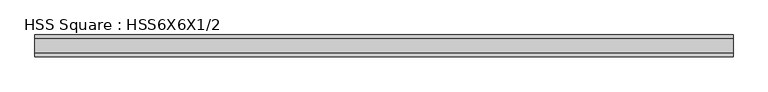
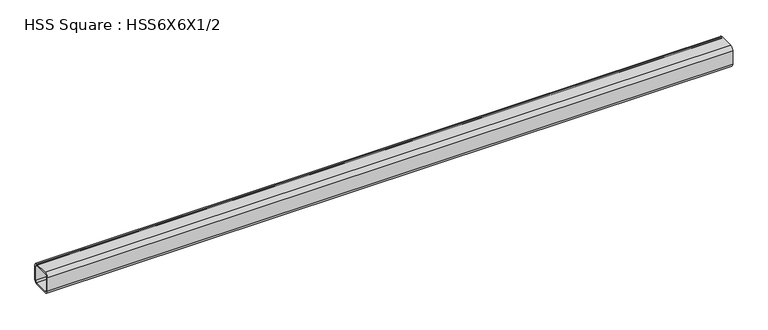
"""IFC4 building model written with IfcOpenShell, lengths in millimetres: member geometry, HSS Square : HSS6X6X1/2."""

from ifc_helpers import new_model, si_unit, point, frame, frame_2d, origin, place, context, project, spatial, polyline, circle_curve, trimmed, segment, composite_curve, outline, extrude, source, transform, mapped, element, save


def hss_square_hss6x6x1_2_5f011b37(model_context):
    return source(origin(), model_context, "Body", "SweptSolid", [
        extrude(outline(composite_curve([segment(trimmed(circle_curve(frame_2d((-50.8, 50.8)), 25.4), [point((-76.2, 50.8))], [point((-50.8, 76.2))], False, "CARTESIAN"), True, "CONTINUOUS"), segment(polyline([(-50.8, 76.2), (50.8, 76.2)]), True, "CONTINUOUS"), segment(trimmed(circle_curve(frame_2d((50.8, 50.8)), 25.4), [point((50.8, 76.2))], [point((76.2, 50.8))], False, "CARTESIAN"), True, "CONTINUOUS"), segment(polyline([(76.2, 50.8), (76.2, -50.8)]), True, "CONTINUOUS"), segment(trimmed(circle_curve(frame_2d((50.8, -50.8)), 25.4), [point((76.2, -50.8))], [point((50.8, -76.2))], False, "CARTESIAN"), True, "CONTINUOUS"), segment(polyline([(50.8, -76.2), (-50.8, -76.2)]), True, "CONTINUOUS"), segment(trimmed(circle_curve(frame_2d((-50.8, -50.8)), 25.4), [point((-50.8, -76.2))], [point((-76.2, -50.8))], False, "CARTESIAN"), True, "CONTINUOUS"), segment(polyline([(-76.2, -50.8), (-76.2, 50.8)]), True, "CONTINUOUS")], self_intersect=False), holes=[composite_curve([segment(polyline([(50.8, 63.5), (-50.8, 63.5)]), True, "CONTINUOUS"), segment(trimmed(circle_curve(frame_2d((-50.8, 50.8)), 12.7), [point((-50.8, 63.5))], [point((-63.5, 50.8))], True, "CARTESIAN"), True, "CONTINUOUS"), segment(polyline([(-63.5, 50.8), (-63.5, -50.8)]), True, "CONTINUOUS"), segment(trimmed(circle_curve(frame_2d((-50.8, -50.8)), 12.7), [point((-63.5, -50.8))], [point((-50.8, -63.5))], True, "CARTESIAN"), True, "CONTINUOUS"), segment(polyline([(-50.8, -63.5), (50.8, -63.5)]), True, "CONTINUOUS"), segment(trimmed(circle_curve(frame_2d((50.8, -50.8)), 12.7), [point((50.8, -63.5))], [point((63.5, -50.8))], True, "CARTESIAN"), True, "CONTINUOUS"), segment(polyline([(63.5, -50.8), (63.5, 50.8)]), True, "CONTINUOUS"), segment(trimmed(circle_curve(frame_2d((50.8, 50.8)), 12.7), [point((63.5, 50.8))], [point((50.8, 63.5))], True, "CARTESIAN"), True, "CONTINUOUS")], self_intersect=False)]), frame((-2376.9834929, 0.0, 0.0), z_axis=(1.0, 0.0, 0.0), x_axis=(0.0, 1.0, 0.0)), (0.0, 0.0, 1.0), 4840.8896454),
    ])


if __name__ == "__main__":
    model = new_model("IFC4")
    model_context = context("Model", 3, world=origin())
    ifc_project = project(units=[si_unit("LENGTHUNIT", "METRE", prefix="MILLI")], contexts=[model_context])
    site = spatial("IfcSite", under=ifc_project)
    building = spatial("IfcBuilding", under=site)
    placement = place(None, origin())
    hss_square_hss6x6x1_2_shape = hss_square_hss6x6x1_2_5f011b37(model_context)
    element("IfcMember", 1, ObjectType="HSS Square : HSS6X6X1/2", at=placement, inside=building, context=model_context, shape_type="MappedRepresentation", body=[
        mapped(hss_square_hss6x6x1_2_shape, transform((0.0, 0.0, 0.0), x_axis=(1.0, 0.0, 0.0), y_axis=(0.0, 1.0, 0.0), z_axis=(0.0, 0.0, 1.0))),
    ])
    save(model, "model.ifc")

# Revit data of these elements
# Type "HSS Square : HSS6X6X1/2"
#   Section Name Key = "HSS 6X6X1/2"
#   Assembly Code = "B10"
#   Width = 6.000"
#   Wall Nominal Thickness = 0.500"
#   Wall Design Thickness = 0.465"
#   Torsional Moment of Inertia = 81.10 in⁴
#   Torsional Modulus = 28.10 in³
#   Section Area = 9.74 in²
#   Plastic Modulus weak axis = 19.80 in³
#   Plastic Modulus strong axis = 19.80 in³
#   Outer Fillet = 1.000"
#   Nominal Weight = 35.24 lbf/ft
#   Moment of Inertia weak axis = 48.30 in⁴
#   Moment of Inertia strong axis = 48.30 in⁴
#   Inner Fillet = 0.500"
#   Height = 6.000"
#   Elastic Modulus weak axis = 16.10 in³
#   Elastic Modulus strong axis = 16.10 in³
#   Centroid Vertical = 3.000"
#   Centroid Horizontal = 3.000"
#   Length [instance default] = 5' - 0"
#   Structural Material [instance default] = Steel ASTM A500, Grade B, Rectangular and Square
#   Principal Axes Angle = 0
# Element 1 (IfcMember, "HSS Square : HSS6X6X1/2")
#   Structural Material = Steel ASTM A992
#   Materials on its faces: "Steel ASTM A992"
# Materials
#   "Steel ASTM A500, Grade B, Rectangular and Square": class "Metal", colour RGB 199 199 199, transparency 0, Description = "Carbon steel", Cost = 0
#   "Steel ASTM A992": class "Metal", colour RGB 199 199 199, transparency 0, Description = "Structural steel 50ksi", Cost = 0
